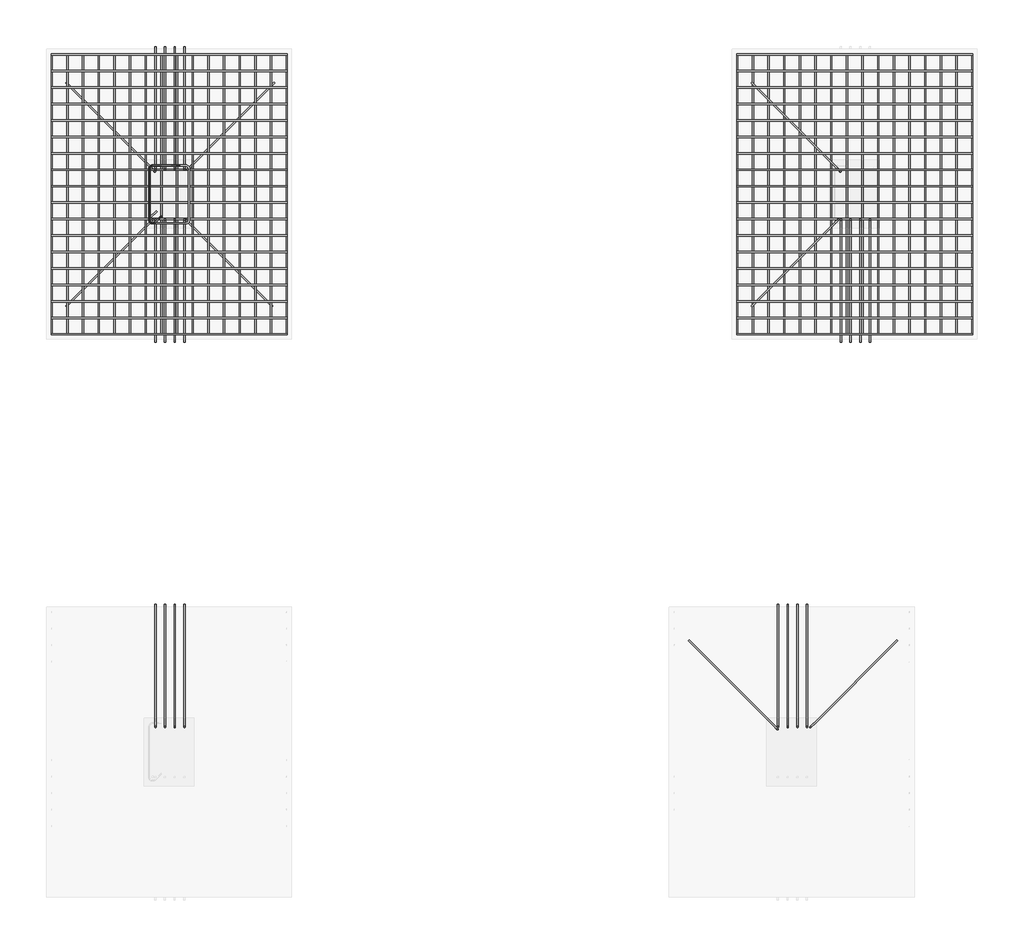
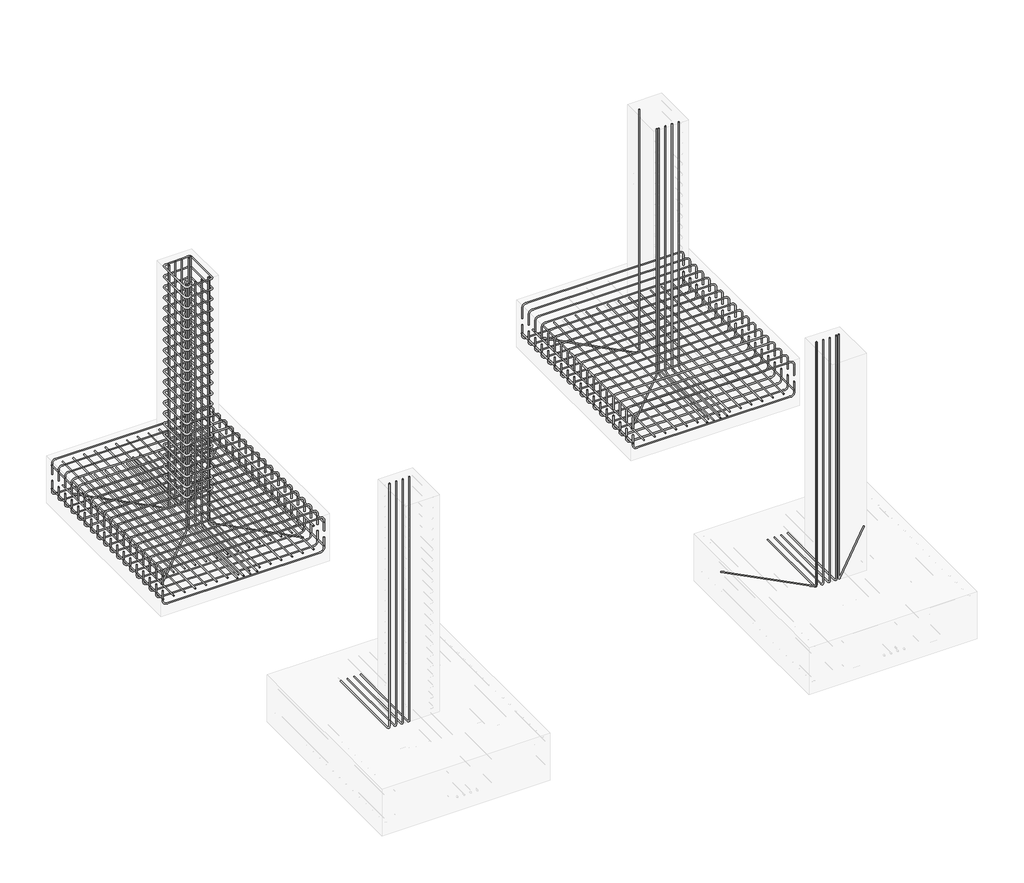
# One storey, part 12 of 33: 21 reinforcing bars.
"""IFC4 building model written with IfcOpenShell, lengths in millimetres."""

from ifc_helpers import new_model, si_unit, point, frame, origin, place, context, project, spatial, polyline, circle_curve, trimmed, segment, composite_curve, source, transform, mapped, element, save
from ifc_brep_helpers import swept_disk

model = new_model("IFC4")

# Units and contexts
model_context = context("Model", 3, world=origin())
ifc_project = project(units=[si_unit("LENGTHUNIT", "METRE", prefix="MILLI")], contexts=[model_context])

# Site, building, storey
site = spatial("IfcSite", under=ifc_project)
building = spatial("IfcBuilding", under=site)
storey = spatial("IfcBuildingStorey", under=building, Elevation=-3000.0)

# Reinforcing bars
placement = place(None, origin())
reinforcing_bar_shape = source(origin(), model_context, "Body", "SolidModel", [
    swept_disk(composite_curve([segment(polyline([(25452.7737106, -2044.0608134, -3240.0), (25452.7737106, -2044.0608134, -3092.7)]), True, "CONTINUOUS"), segment(trimmed(circle_curve(frame((25499.1237106, -2044.0608134, -3092.7), z_axis=(0.0, 1.0, 0.0), x_axis=(-46.35000000000218, 0.0, 0.0)), 46.35), [point((25452.7737106, -2044.0608134, -3092.7))], [point((25499.1237106, -2044.0608134, -3046.35))], True, "CARTESIAN"), True, "CONTINUOUS"), segment(polyline([(25499.1237106, -2044.0608134, -3046.35), (27513.7237106, -2044.0608134, -3046.35)]), True, "CONTINUOUS"), segment(trimmed(circle_curve(frame((27513.7237106, -2044.0608134, -3092.7), z_axis=(0.0, 1.0, 0.0), x_axis=(0.0, 0.0, 46.34999999999991)), 46.35), [point((27513.7237106, -2044.0608134, -3046.35))], [point((27560.0737106, -2044.0608134, -3092.7))], True, "CARTESIAN"), True, "CONTINUOUS"), segment(polyline([(27560.0737106, -2044.0608134, -3092.7), (27560.0737106, -2044.0608134, -3240.0)]), True, "CONTINUOUS")], self_intersect=False), 6.35),
])
element("IfcReinforcingBar", 1, at=placement, inside=storey, context=model_context, shape_type="MappedRepresentation", body=[
    mapped(reinforcing_bar_shape, transform((0.0, 0.0, 0.0), x_axis=(1.0, 0.0, 0.0), y_axis=(0.0, 1.0, 0.0), z_axis=(0.0, 0.0, 1.0))),
    mapped(reinforcing_bar_shape, transform((0.0, -147.4882353, 0.0), x_axis=(1.0, 0.0, 0.0), y_axis=(0.0, 1.0, 0.0), z_axis=(0.0, 0.0, 1.0))),
    mapped(reinforcing_bar_shape, transform((0.0, -294.9764706, 0.0), x_axis=(1.0, 0.0, 0.0), y_axis=(0.0, 1.0, 0.0), z_axis=(0.0, 0.0, 1.0))),
    mapped(reinforcing_bar_shape, transform((0.0, -442.4647059, 0.0), x_axis=(1.0, 0.0, 0.0), y_axis=(0.0, 1.0, 0.0), z_axis=(0.0, 0.0, 1.0))),
    mapped(reinforcing_bar_shape, transform((0.0, -589.9529412, 0.0), x_axis=(1.0, 0.0, 0.0), y_axis=(0.0, 1.0, 0.0), z_axis=(0.0, 0.0, 1.0))),
    mapped(reinforcing_bar_shape, transform((0.0, -737.4411765, 0.0), x_axis=(1.0, 0.0, 0.0), y_axis=(0.0, 1.0, 0.0), z_axis=(0.0, 0.0, 1.0))),
    mapped(reinforcing_bar_shape, transform((0.0, -884.9294118, 0.0), x_axis=(1.0, 0.0, 0.0), y_axis=(0.0, 1.0, 0.0), z_axis=(0.0, 0.0, 1.0))),
    mapped(reinforcing_bar_shape, transform((0.0, -1032.4176471, 0.0), x_axis=(1.0, 0.0, 0.0), y_axis=(0.0, 1.0, 0.0), z_axis=(0.0, 0.0, 1.0))),
    mapped(reinforcing_bar_shape, transform((0.0, -1179.9058824, 0.0), x_axis=(1.0, 0.0, 0.0), y_axis=(0.0, 1.0, 0.0), z_axis=(0.0, 0.0, 1.0))),
    mapped(reinforcing_bar_shape, transform((0.0, -1327.3941176, 0.0), x_axis=(1.0, 0.0, 0.0), y_axis=(0.0, 1.0, 0.0), z_axis=(0.0, 0.0, 1.0))),
    mapped(reinforcing_bar_shape, transform((0.0, -1474.8823529, 0.0), x_axis=(1.0, 0.0, 0.0), y_axis=(0.0, 1.0, 0.0), z_axis=(0.0, 0.0, 1.0))),
    mapped(reinforcing_bar_shape, transform((0.0, -1622.3705882, 0.0), x_axis=(1.0, 0.0, 0.0), y_axis=(0.0, 1.0, 0.0), z_axis=(0.0, 0.0, 1.0))),
    mapped(reinforcing_bar_shape, transform((0.0, -1769.8588235, 0.0), x_axis=(1.0, 0.0, 0.0), y_axis=(0.0, 1.0, 0.0), z_axis=(0.0, 0.0, 1.0))),
    mapped(reinforcing_bar_shape, transform((0.0, -1917.3470588, 0.0), x_axis=(1.0, 0.0, 0.0), y_axis=(0.0, 1.0, 0.0), z_axis=(0.0, 0.0, 1.0))),
    mapped(reinforcing_bar_shape, transform((0.0, -2064.8352941, 0.0), x_axis=(1.0, 0.0, 0.0), y_axis=(0.0, 1.0, 0.0), z_axis=(0.0, 0.0, 1.0))),
    mapped(reinforcing_bar_shape, transform((0.0, -2212.3235294, 0.0), x_axis=(1.0, 0.0, 0.0), y_axis=(0.0, 1.0, 0.0), z_axis=(0.0, 0.0, 1.0))),
    mapped(reinforcing_bar_shape, transform((0.0, -2359.8117647, 0.0), x_axis=(1.0, 0.0, 0.0), y_axis=(0.0, 1.0, 0.0), z_axis=(0.0, 0.0, 1.0))),
    mapped(reinforcing_bar_shape, transform((0.0, -2507.3, 0.0), x_axis=(1.0, 0.0, 0.0), y_axis=(0.0, 1.0, 0.0), z_axis=(0.0, 0.0, 1.0))),
])
reinforcing_bar_2_shape = source(origin(), model_context, "Body", "SolidModel", [
    swept_disk(composite_curve([segment(polyline([(27560.0737106, -2044.0608134, -3330.080452), (27560.0737106, -2044.0608134, -3477.380452)]), True, "CONTINUOUS"), segment(trimmed(circle_curve(frame((27513.7237106, -2044.0608134, -3477.380452), z_axis=(0.0, 1.0, 0.0), x_axis=(46.35000000000218, 0.0, 0.0)), 46.35), [point((27560.0737106, -2044.0608134, -3477.380452))], [point((27513.7237106, -2044.0608134, -3523.730452))], True, "CARTESIAN"), True, "CONTINUOUS"), segment(polyline([(27513.7237106, -2044.0608134, -3523.730452), (25499.1237106, -2044.0608134, -3523.730452)]), True, "CONTINUOUS"), segment(trimmed(circle_curve(frame((25499.1237106, -2044.0608134, -3477.380452), z_axis=(0.0, 1.0, 0.0), x_axis=(0.0, 0.0, -46.34999999999991)), 46.35), [point((25499.1237106, -2044.0608134, -3523.730452))], [point((25452.7737106, -2044.0608134, -3477.380452))], True, "CARTESIAN"), True, "CONTINUOUS"), segment(polyline([(25452.7737106, -2044.0608134, -3477.380452), (25452.7737106, -2044.0608134, -3330.080452)]), True, "CONTINUOUS")], self_intersect=False), 6.35),
])
element("IfcReinforcingBar", 2, at=placement, inside=storey, context=model_context, shape_type="MappedRepresentation", body=[
    mapped(reinforcing_bar_2_shape, transform((0.0, 0.0, 0.0), x_axis=(1.0, 0.0, 0.0), y_axis=(0.0, 1.0, 0.0), z_axis=(0.0, 0.0, 1.0))),
    mapped(reinforcing_bar_2_shape, transform((0.0, -147.4882353, 0.0), x_axis=(1.0, 0.0, 0.0), y_axis=(0.0, 1.0, 0.0), z_axis=(0.0, 0.0, 1.0))),
    mapped(reinforcing_bar_2_shape, transform((0.0, -294.9764706, 0.0), x_axis=(1.0, 0.0, 0.0), y_axis=(0.0, 1.0, 0.0), z_axis=(0.0, 0.0, 1.0))),
    mapped(reinforcing_bar_2_shape, transform((0.0, -442.4647059, 0.0), x_axis=(1.0, 0.0, 0.0), y_axis=(0.0, 1.0, 0.0), z_axis=(0.0, 0.0, 1.0))),
    mapped(reinforcing_bar_2_shape, transform((0.0, -589.9529412, 0.0), x_axis=(1.0, 0.0, 0.0), y_axis=(0.0, 1.0, 0.0), z_axis=(0.0, 0.0, 1.0))),
    mapped(reinforcing_bar_2_shape, transform((0.0, -737.4411765, 0.0), x_axis=(1.0, 0.0, 0.0), y_axis=(0.0, 1.0, 0.0), z_axis=(0.0, 0.0, 1.0))),
    mapped(reinforcing_bar_2_shape, transform((0.0, -884.9294118, 0.0), x_axis=(1.0, 0.0, 0.0), y_axis=(0.0, 1.0, 0.0), z_axis=(0.0, 0.0, 1.0))),
    mapped(reinforcing_bar_2_shape, transform((0.0, -1032.4176471, 0.0), x_axis=(1.0, 0.0, 0.0), y_axis=(0.0, 1.0, 0.0), z_axis=(0.0, 0.0, 1.0))),
    mapped(reinforcing_bar_2_shape, transform((0.0, -1179.9058824, 0.0), x_axis=(1.0, 0.0, 0.0), y_axis=(0.0, 1.0, 0.0), z_axis=(0.0, 0.0, 1.0))),
    mapped(reinforcing_bar_2_shape, transform((0.0, -1327.3941176, 0.0), x_axis=(1.0, 0.0, 0.0), y_axis=(0.0, 1.0, 0.0), z_axis=(0.0, 0.0, 1.0))),
    mapped(reinforcing_bar_2_shape, transform((0.0, -1474.8823529, 0.0), x_axis=(1.0, 0.0, 0.0), y_axis=(0.0, 1.0, 0.0), z_axis=(0.0, 0.0, 1.0))),
    mapped(reinforcing_bar_2_shape, transform((0.0, -1622.3705882, 0.0), x_axis=(1.0, 0.0, 0.0), y_axis=(0.0, 1.0, 0.0), z_axis=(0.0, 0.0, 1.0))),
    mapped(reinforcing_bar_2_shape, transform((0.0, -1769.8588235, 0.0), x_axis=(1.0, 0.0, 0.0), y_axis=(0.0, 1.0, 0.0), z_axis=(0.0, 0.0, 1.0))),
    mapped(reinforcing_bar_2_shape, transform((0.0, -1917.3470588, 0.0), x_axis=(1.0, 0.0, 0.0), y_axis=(0.0, 1.0, 0.0), z_axis=(0.0, 0.0, 1.0))),
    mapped(reinforcing_bar_2_shape, transform((0.0, -2064.8352941, 0.0), x_axis=(1.0, 0.0, 0.0), y_axis=(0.0, 1.0, 0.0), z_axis=(0.0, 0.0, 1.0))),
    mapped(reinforcing_bar_2_shape, transform((0.0, -2212.3235294, 0.0), x_axis=(1.0, 0.0, 0.0), y_axis=(0.0, 1.0, 0.0), z_axis=(0.0, 0.0, 1.0))),
    mapped(reinforcing_bar_2_shape, transform((0.0, -2359.8117647, 0.0), x_axis=(1.0, 0.0, 0.0), y_axis=(0.0, 1.0, 0.0), z_axis=(0.0, 0.0, 1.0))),
    mapped(reinforcing_bar_2_shape, transform((0.0, -2507.3, 0.0), x_axis=(1.0, 0.0, 0.0), y_axis=(0.0, 1.0, 0.0), z_axis=(0.0, 0.0, 1.0))),
])
reinforcing_bar_3_shape = source(origin(), model_context, "Body", "SolidModel", [
    swept_disk(composite_curve([segment(polyline([(27560.0737106, -4557.7108134, -3447.8614173), (27560.0737106, -2037.7108134, -3447.8614173)]), True, "CONTINUOUS")], self_intersect=False), 6.35),
])
element("IfcReinforcingBar", 3, at=placement, inside=storey, context=model_context, shape_type="MappedRepresentation", body=[
    mapped(reinforcing_bar_3_shape, transform((0.0, 0.0, 0.0), x_axis=(1.0, 0.0, 0.0), y_axis=(0.0, 1.0, 0.0), z_axis=(0.0, 0.0, 1.0))),
    mapped(reinforcing_bar_3_shape, transform((-140.4866667, 0.0, 0.0), x_axis=(1.0, 0.0, 0.0), y_axis=(0.0, 1.0, 0.0), z_axis=(0.0, 0.0, 1.0))),
    mapped(reinforcing_bar_3_shape, transform((-280.9733333, 0.0, 0.0), x_axis=(1.0, 0.0, 0.0), y_axis=(0.0, 1.0, 0.0), z_axis=(0.0, 0.0, 1.0))),
    mapped(reinforcing_bar_3_shape, transform((-421.46, 0.0, 0.0), x_axis=(1.0, 0.0, 0.0), y_axis=(0.0, 1.0, 0.0), z_axis=(0.0, 0.0, 1.0))),
    mapped(reinforcing_bar_3_shape, transform((-561.9466667, 0.0, 0.0), x_axis=(1.0, 0.0, 0.0), y_axis=(0.0, 1.0, 0.0), z_axis=(0.0, 0.0, 1.0))),
    mapped(reinforcing_bar_3_shape, transform((-702.4333333, 0.0, 0.0), x_axis=(1.0, 0.0, 0.0), y_axis=(0.0, 1.0, 0.0), z_axis=(0.0, 0.0, 1.0))),
    mapped(reinforcing_bar_3_shape, transform((-842.92, 0.0, 0.0), x_axis=(1.0, 0.0, 0.0), y_axis=(0.0, 1.0, 0.0), z_axis=(0.0, 0.0, 1.0))),
    mapped(reinforcing_bar_3_shape, transform((-983.4066667, 0.0, 0.0), x_axis=(1.0, 0.0, 0.0), y_axis=(0.0, 1.0, 0.0), z_axis=(0.0, 0.0, 1.0))),
    mapped(reinforcing_bar_3_shape, transform((-1123.8933333, 0.0, 0.0), x_axis=(1.0, 0.0, 0.0), y_axis=(0.0, 1.0, 0.0), z_axis=(0.0, 0.0, 1.0))),
    mapped(reinforcing_bar_3_shape, transform((-1264.38, 0.0, 0.0), x_axis=(1.0, 0.0, 0.0), y_axis=(0.0, 1.0, 0.0), z_axis=(0.0, 0.0, 1.0))),
    mapped(reinforcing_bar_3_shape, transform((-1404.8666667, 0.0, 0.0), x_axis=(1.0, 0.0, 0.0), y_axis=(0.0, 1.0, 0.0), z_axis=(0.0, 0.0, 1.0))),
    mapped(reinforcing_bar_3_shape, transform((-1545.3533333, 0.0, 0.0), x_axis=(1.0, 0.0, 0.0), y_axis=(0.0, 1.0, 0.0), z_axis=(0.0, 0.0, 1.0))),
    mapped(reinforcing_bar_3_shape, transform((-1685.84, 0.0, 0.0), x_axis=(1.0, 0.0, 0.0), y_axis=(0.0, 1.0, 0.0), z_axis=(0.0, 0.0, 1.0))),
    mapped(reinforcing_bar_3_shape, transform((-1826.3266667, 0.0, 0.0), x_axis=(1.0, 0.0, 0.0), y_axis=(0.0, 1.0, 0.0), z_axis=(0.0, 0.0, 1.0))),
    mapped(reinforcing_bar_3_shape, transform((-1966.8133333, 0.0, 0.0), x_axis=(1.0, 0.0, 0.0), y_axis=(0.0, 1.0, 0.0), z_axis=(0.0, 0.0, 1.0))),
    mapped(reinforcing_bar_3_shape, transform((-2107.3, 0.0, 0.0), x_axis=(1.0, 0.0, 0.0), y_axis=(0.0, 1.0, 0.0), z_axis=(0.0, 0.0, 1.0))),
])
reinforcing_bar_4_shape = source(origin(), model_context, "Body", "SolidModel", [
    swept_disk(composite_curve([segment(polyline([(19306.5357258, -2044.0608134, -3240.0), (19306.5357258, -2044.0608134, -3092.7)]), True, "CONTINUOUS"), segment(trimmed(circle_curve(frame((19352.8857258, -2044.0608134, -3092.7), z_axis=(0.0, 1.0, 0.0), x_axis=(-46.349999999998545, 0.0, 0.0)), 46.35), [point((19306.5357258, -2044.0608134, -3092.7))], [point((19352.8857258, -2044.0608134, -3046.35))], True, "CARTESIAN"), True, "CONTINUOUS"), segment(polyline([(19352.8857258, -2044.0608134, -3046.35), (21367.4857258, -2044.0608134, -3046.35)]), True, "CONTINUOUS"), segment(trimmed(circle_curve(frame((21367.4857258, -2044.0608134, -3092.7), z_axis=(0.0, 1.0, 0.0), x_axis=(0.0, 0.0, 46.34999999999991)), 46.35), [point((21367.4857258, -2044.0608134, -3046.35))], [point((21413.8357258, -2044.0608134, -3092.7))], True, "CARTESIAN"), True, "CONTINUOUS"), segment(polyline([(21413.8357258, -2044.0608134, -3092.7), (21413.8357258, -2044.0608134, -3240.0)]), True, "CONTINUOUS")], self_intersect=False), 6.35),
])
element("IfcReinforcingBar", 4, at=placement, inside=storey, context=model_context, shape_type="MappedRepresentation", body=[
    mapped(reinforcing_bar_4_shape, transform((0.0, 0.0, 0.0), x_axis=(1.0, 0.0, 0.0), y_axis=(0.0, 1.0, 0.0), z_axis=(0.0, 0.0, 1.0))),
    mapped(reinforcing_bar_4_shape, transform((0.0, -147.4882353, 0.0), x_axis=(1.0, 0.0, 0.0), y_axis=(0.0, 1.0, 0.0), z_axis=(0.0, 0.0, 1.0))),
    mapped(reinforcing_bar_4_shape, transform((0.0, -294.9764706, 0.0), x_axis=(1.0, 0.0, 0.0), y_axis=(0.0, 1.0, 0.0), z_axis=(0.0, 0.0, 1.0))),
    mapped(reinforcing_bar_4_shape, transform((0.0, -442.4647059, 0.0), x_axis=(1.0, 0.0, 0.0), y_axis=(0.0, 1.0, 0.0), z_axis=(0.0, 0.0, 1.0))),
    mapped(reinforcing_bar_4_shape, transform((0.0, -589.9529412, 0.0), x_axis=(1.0, 0.0, 0.0), y_axis=(0.0, 1.0, 0.0), z_axis=(0.0, 0.0, 1.0))),
    mapped(reinforcing_bar_4_shape, transform((0.0, -737.4411765, 0.0), x_axis=(1.0, 0.0, 0.0), y_axis=(0.0, 1.0, 0.0), z_axis=(0.0, 0.0, 1.0))),
    mapped(reinforcing_bar_4_shape, transform((0.0, -884.9294118, 0.0), x_axis=(1.0, 0.0, 0.0), y_axis=(0.0, 1.0, 0.0), z_axis=(0.0, 0.0, 1.0))),
    mapped(reinforcing_bar_4_shape, transform((0.0, -1032.4176471, 0.0), x_axis=(1.0, 0.0, 0.0), y_axis=(0.0, 1.0, 0.0), z_axis=(0.0, 0.0, 1.0))),
    mapped(reinforcing_bar_4_shape, transform((0.0, -1179.9058824, 0.0), x_axis=(1.0, 0.0, 0.0), y_axis=(0.0, 1.0, 0.0), z_axis=(0.0, 0.0, 1.0))),
    mapped(reinforcing_bar_4_shape, transform((0.0, -1327.3941176, 0.0), x_axis=(1.0, 0.0, 0.0), y_axis=(0.0, 1.0, 0.0), z_axis=(0.0, 0.0, 1.0))),
    mapped(reinforcing_bar_4_shape, transform((0.0, -1474.8823529, 0.0), x_axis=(1.0, 0.0, 0.0), y_axis=(0.0, 1.0, 0.0), z_axis=(0.0, 0.0, 1.0))),
    mapped(reinforcing_bar_4_shape, transform((0.0, -1622.3705882, 0.0), x_axis=(1.0, 0.0, 0.0), y_axis=(0.0, 1.0, 0.0), z_axis=(0.0, 0.0, 1.0))),
    mapped(reinforcing_bar_4_shape, transform((0.0, -1769.8588235, 0.0), x_axis=(1.0, 0.0, 0.0), y_axis=(0.0, 1.0, 0.0), z_axis=(0.0, 0.0, 1.0))),
    mapped(reinforcing_bar_4_shape, transform((0.0, -1917.3470588, 0.0), x_axis=(1.0, 0.0, 0.0), y_axis=(0.0, 1.0, 0.0), z_axis=(0.0, 0.0, 1.0))),
    mapped(reinforcing_bar_4_shape, transform((0.0, -2064.8352941, 0.0), x_axis=(1.0, 0.0, 0.0), y_axis=(0.0, 1.0, 0.0), z_axis=(0.0, 0.0, 1.0))),
    mapped(reinforcing_bar_4_shape, transform((0.0, -2212.3235294, 0.0), x_axis=(1.0, 0.0, 0.0), y_axis=(0.0, 1.0, 0.0), z_axis=(0.0, 0.0, 1.0))),
    mapped(reinforcing_bar_4_shape, transform((0.0, -2359.8117647, 0.0), x_axis=(1.0, 0.0, 0.0), y_axis=(0.0, 1.0, 0.0), z_axis=(0.0, 0.0, 1.0))),
    mapped(reinforcing_bar_4_shape, transform((0.0, -2507.3, 0.0), x_axis=(1.0, 0.0, 0.0), y_axis=(0.0, 1.0, 0.0), z_axis=(0.0, 0.0, 1.0))),
])
reinforcing_bar_5_shape = source(origin(), model_context, "Body", "SolidModel", [
    swept_disk(composite_curve([segment(polyline([(21413.8357258, -2044.0608134, -3330.080452), (21413.8357258, -2044.0608134, -3477.380452)]), True, "CONTINUOUS"), segment(trimmed(circle_curve(frame((21367.4857258, -2044.0608134, -3477.380452), z_axis=(0.0, 1.0, 0.0), x_axis=(46.349999999998545, 0.0, 0.0)), 46.35), [point((21413.8357258, -2044.0608134, -3477.380452))], [point((21367.4857258, -2044.0608134, -3523.730452))], True, "CARTESIAN"), True, "CONTINUOUS"), segment(polyline([(21367.4857258, -2044.0608134, -3523.730452), (19352.8857258, -2044.0608134, -3523.730452)]), True, "CONTINUOUS"), segment(trimmed(circle_curve(frame((19352.8857258, -2044.0608134, -3477.380452), z_axis=(0.0, 1.0, 0.0), x_axis=(0.0, 0.0, -46.34999999999991)), 46.35), [point((19352.8857258, -2044.0608134, -3523.730452))], [point((19306.5357258, -2044.0608134, -3477.380452))], True, "CARTESIAN"), True, "CONTINUOUS"), segment(polyline([(19306.5357258, -2044.0608134, -3477.380452), (19306.5357258, -2044.0608134, -3330.080452)]), True, "CONTINUOUS")], self_intersect=False), 6.35),
])
element("IfcReinforcingBar", 5, at=placement, inside=storey, context=model_context, shape_type="MappedRepresentation", body=[
    mapped(reinforcing_bar_5_shape, transform((0.0, 0.0, 0.0), x_axis=(1.0, 0.0, 0.0), y_axis=(0.0, 1.0, 0.0), z_axis=(0.0, 0.0, 1.0))),
    mapped(reinforcing_bar_5_shape, transform((0.0, -147.4882353, 0.0), x_axis=(1.0, 0.0, 0.0), y_axis=(0.0, 1.0, 0.0), z_axis=(0.0, 0.0, 1.0))),
    mapped(reinforcing_bar_5_shape, transform((0.0, -294.9764706, 0.0), x_axis=(1.0, 0.0, 0.0), y_axis=(0.0, 1.0, 0.0), z_axis=(0.0, 0.0, 1.0))),
    mapped(reinforcing_bar_5_shape, transform((0.0, -442.4647059, 0.0), x_axis=(1.0, 0.0, 0.0), y_axis=(0.0, 1.0, 0.0), z_axis=(0.0, 0.0, 1.0))),
    mapped(reinforcing_bar_5_shape, transform((0.0, -589.9529412, 0.0), x_axis=(1.0, 0.0, 0.0), y_axis=(0.0, 1.0, 0.0), z_axis=(0.0, 0.0, 1.0))),
    mapped(reinforcing_bar_5_shape, transform((0.0, -737.4411765, 0.0), x_axis=(1.0, 0.0, 0.0), y_axis=(0.0, 1.0, 0.0), z_axis=(0.0, 0.0, 1.0))),
    mapped(reinforcing_bar_5_shape, transform((0.0, -884.9294118, 0.0), x_axis=(1.0, 0.0, 0.0), y_axis=(0.0, 1.0, 0.0), z_axis=(0.0, 0.0, 1.0))),
    mapped(reinforcing_bar_5_shape, transform((0.0, -1032.4176471, 0.0), x_axis=(1.0, 0.0, 0.0), y_axis=(0.0, 1.0, 0.0), z_axis=(0.0, 0.0, 1.0))),
    mapped(reinforcing_bar_5_shape, transform((0.0, -1179.9058824, 0.0), x_axis=(1.0, 0.0, 0.0), y_axis=(0.0, 1.0, 0.0), z_axis=(0.0, 0.0, 1.0))),
    mapped(reinforcing_bar_5_shape, transform((0.0, -1327.3941176, 0.0), x_axis=(1.0, 0.0, 0.0), y_axis=(0.0, 1.0, 0.0), z_axis=(0.0, 0.0, 1.0))),
    mapped(reinforcing_bar_5_shape, transform((0.0, -1474.8823529, 0.0), x_axis=(1.0, 0.0, 0.0), y_axis=(0.0, 1.0, 0.0), z_axis=(0.0, 0.0, 1.0))),
    mapped(reinforcing_bar_5_shape, transform((0.0, -1622.3705882, 0.0), x_axis=(1.0, 0.0, 0.0), y_axis=(0.0, 1.0, 0.0), z_axis=(0.0, 0.0, 1.0))),
    mapped(reinforcing_bar_5_shape, transform((0.0, -1769.8588235, 0.0), x_axis=(1.0, 0.0, 0.0), y_axis=(0.0, 1.0, 0.0), z_axis=(0.0, 0.0, 1.0))),
    mapped(reinforcing_bar_5_shape, transform((0.0, -1917.3470588, 0.0), x_axis=(1.0, 0.0, 0.0), y_axis=(0.0, 1.0, 0.0), z_axis=(0.0, 0.0, 1.0))),
    mapped(reinforcing_bar_5_shape, transform((0.0, -2064.8352941, 0.0), x_axis=(1.0, 0.0, 0.0), y_axis=(0.0, 1.0, 0.0), z_axis=(0.0, 0.0, 1.0))),
    mapped(reinforcing_bar_5_shape, transform((0.0, -2212.3235294, 0.0), x_axis=(1.0, 0.0, 0.0), y_axis=(0.0, 1.0, 0.0), z_axis=(0.0, 0.0, 1.0))),
    mapped(reinforcing_bar_5_shape, transform((0.0, -2359.8117647, 0.0), x_axis=(1.0, 0.0, 0.0), y_axis=(0.0, 1.0, 0.0), z_axis=(0.0, 0.0, 1.0))),
    mapped(reinforcing_bar_5_shape, transform((0.0, -2507.3, 0.0), x_axis=(1.0, 0.0, 0.0), y_axis=(0.0, 1.0, 0.0), z_axis=(0.0, 0.0, 1.0))),
])
reinforcing_bar_6_shape = source(origin(), model_context, "Body", "SolidModel", [
    swept_disk(composite_curve([segment(polyline([(21413.8357258, -4557.7108134, -3447.8614173), (21413.8357258, -2037.7108134, -3447.8614173)]), True, "CONTINUOUS")], self_intersect=False), 6.35),
])
element("IfcReinforcingBar", 6, at=placement, inside=storey, context=model_context, shape_type="MappedRepresentation", body=[
    mapped(reinforcing_bar_6_shape, transform((0.0, 0.0, 0.0), x_axis=(1.0, 0.0, 0.0), y_axis=(0.0, 1.0, 0.0), z_axis=(0.0, 0.0, 1.0))),
    mapped(reinforcing_bar_6_shape, transform((-140.4866667, 0.0, 0.0), x_axis=(1.0, 0.0, 0.0), y_axis=(0.0, 1.0, 0.0), z_axis=(0.0, 0.0, 1.0))),
    mapped(reinforcing_bar_6_shape, transform((-280.9733333, 0.0, 0.0), x_axis=(1.0, 0.0, 0.0), y_axis=(0.0, 1.0, 0.0), z_axis=(0.0, 0.0, 1.0))),
    mapped(reinforcing_bar_6_shape, transform((-421.46, 0.0, 0.0), x_axis=(1.0, 0.0, 0.0), y_axis=(0.0, 1.0, 0.0), z_axis=(0.0, 0.0, 1.0))),
    mapped(reinforcing_bar_6_shape, transform((-561.9466667, 0.0, 0.0), x_axis=(1.0, 0.0, 0.0), y_axis=(0.0, 1.0, 0.0), z_axis=(0.0, 0.0, 1.0))),
    mapped(reinforcing_bar_6_shape, transform((-702.4333333, 0.0, 0.0), x_axis=(1.0, 0.0, 0.0), y_axis=(0.0, 1.0, 0.0), z_axis=(0.0, 0.0, 1.0))),
    mapped(reinforcing_bar_6_shape, transform((-842.92, 0.0, 0.0), x_axis=(1.0, 0.0, 0.0), y_axis=(0.0, 1.0, 0.0), z_axis=(0.0, 0.0, 1.0))),
    mapped(reinforcing_bar_6_shape, transform((-983.4066667, 0.0, 0.0), x_axis=(1.0, 0.0, 0.0), y_axis=(0.0, 1.0, 0.0), z_axis=(0.0, 0.0, 1.0))),
    mapped(reinforcing_bar_6_shape, transform((-1123.8933333, 0.0, 0.0), x_axis=(1.0, 0.0, 0.0), y_axis=(0.0, 1.0, 0.0), z_axis=(0.0, 0.0, 1.0))),
    mapped(reinforcing_bar_6_shape, transform((-1264.38, 0.0, 0.0), x_axis=(1.0, 0.0, 0.0), y_axis=(0.0, 1.0, 0.0), z_axis=(0.0, 0.0, 1.0))),
    mapped(reinforcing_bar_6_shape, transform((-1404.8666667, 0.0, 0.0), x_axis=(1.0, 0.0, 0.0), y_axis=(0.0, 1.0, 0.0), z_axis=(0.0, 0.0, 1.0))),
    mapped(reinforcing_bar_6_shape, transform((-1545.3533333, 0.0, 0.0), x_axis=(1.0, 0.0, 0.0), y_axis=(0.0, 1.0, 0.0), z_axis=(0.0, 0.0, 1.0))),
    mapped(reinforcing_bar_6_shape, transform((-1685.84, 0.0, 0.0), x_axis=(1.0, 0.0, 0.0), y_axis=(0.0, 1.0, 0.0), z_axis=(0.0, 0.0, 1.0))),
    mapped(reinforcing_bar_6_shape, transform((-1826.3266667, 0.0, 0.0), x_axis=(1.0, 0.0, 0.0), y_axis=(0.0, 1.0, 0.0), z_axis=(0.0, 0.0, 1.0))),
    mapped(reinforcing_bar_6_shape, transform((-1966.8133333, 0.0, 0.0), x_axis=(1.0, 0.0, 0.0), y_axis=(0.0, 1.0, 0.0), z_axis=(0.0, 0.0, 1.0))),
    mapped(reinforcing_bar_6_shape, transform((-2107.3, 0.0, 0.0), x_axis=(1.0, 0.0, 0.0), y_axis=(0.0, 1.0, 0.0), z_axis=(0.0, 0.0, 1.0))),
])
reinforcing_bar_7_shape = source(origin(), model_context, "Body", "SolidModel", [
    swept_disk(composite_curve([segment(polyline([(19306.5357258, -4557.7108134, -3122.7084113), (19306.5357258, -2037.7108134, -3122.7084113)]), True, "CONTINUOUS")], self_intersect=False), 6.35),
])
element("IfcReinforcingBar", 7, at=placement, inside=storey, context=model_context, shape_type="MappedRepresentation", body=[
    mapped(reinforcing_bar_7_shape, transform((0.0, 0.0, 0.0), x_axis=(1.0, 0.0, 0.0), y_axis=(0.0, 1.0, 0.0), z_axis=(0.0, 0.0, 1.0))),
    mapped(reinforcing_bar_7_shape, transform((140.4866667, 0.0, 0.0), x_axis=(1.0, 0.0, 0.0), y_axis=(0.0, 1.0, 0.0), z_axis=(0.0, 0.0, 1.0))),
    mapped(reinforcing_bar_7_shape, transform((280.9733333, 0.0, 0.0), x_axis=(1.0, 0.0, 0.0), y_axis=(0.0, 1.0, 0.0), z_axis=(0.0, 0.0, 1.0))),
    mapped(reinforcing_bar_7_shape, transform((421.46, 0.0, 0.0), x_axis=(1.0, 0.0, 0.0), y_axis=(0.0, 1.0, 0.0), z_axis=(0.0, 0.0, 1.0))),
    mapped(reinforcing_bar_7_shape, transform((561.9466667, 0.0, 0.0), x_axis=(1.0, 0.0, 0.0), y_axis=(0.0, 1.0, 0.0), z_axis=(0.0, 0.0, 1.0))),
    mapped(reinforcing_bar_7_shape, transform((702.4333333, 0.0, 0.0), x_axis=(1.0, 0.0, 0.0), y_axis=(0.0, 1.0, 0.0), z_axis=(0.0, 0.0, 1.0))),
    mapped(reinforcing_bar_7_shape, transform((842.92, 0.0, 0.0), x_axis=(1.0, 0.0, 0.0), y_axis=(0.0, 1.0, 0.0), z_axis=(0.0, 0.0, 1.0))),
    mapped(reinforcing_bar_7_shape, transform((983.4066667, 0.0, 0.0), x_axis=(1.0, 0.0, 0.0), y_axis=(0.0, 1.0, 0.0), z_axis=(0.0, 0.0, 1.0))),
    mapped(reinforcing_bar_7_shape, transform((1123.8933333, 0.0, 0.0), x_axis=(1.0, 0.0, 0.0), y_axis=(0.0, 1.0, 0.0), z_axis=(0.0, 0.0, 1.0))),
    mapped(reinforcing_bar_7_shape, transform((1264.38, 0.0, 0.0), x_axis=(1.0, 0.0, 0.0), y_axis=(0.0, 1.0, 0.0), z_axis=(0.0, 0.0, 1.0))),
    mapped(reinforcing_bar_7_shape, transform((1404.8666667, 0.0, 0.0), x_axis=(1.0, 0.0, 0.0), y_axis=(0.0, 1.0, 0.0), z_axis=(0.0, 0.0, 1.0))),
    mapped(reinforcing_bar_7_shape, transform((1545.3533333, 0.0, 0.0), x_axis=(1.0, 0.0, 0.0), y_axis=(0.0, 1.0, 0.0), z_axis=(0.0, 0.0, 1.0))),
    mapped(reinforcing_bar_7_shape, transform((1685.84, 0.0, 0.0), x_axis=(1.0, 0.0, 0.0), y_axis=(0.0, 1.0, 0.0), z_axis=(0.0, 0.0, 1.0))),
    mapped(reinforcing_bar_7_shape, transform((1826.3266667, 0.0, 0.0), x_axis=(1.0, 0.0, 0.0), y_axis=(0.0, 1.0, 0.0), z_axis=(0.0, 0.0, 1.0))),
    mapped(reinforcing_bar_7_shape, transform((1966.8133333, 0.0, 0.0), x_axis=(1.0, 0.0, 0.0), y_axis=(0.0, 1.0, 0.0), z_axis=(0.0, 0.0, 1.0))),
    mapped(reinforcing_bar_7_shape, transform((2107.3, 0.0, 0.0), x_axis=(1.0, 0.0, 0.0), y_axis=(0.0, 1.0, 0.0), z_axis=(0.0, 0.0, 1.0))),
])
reinforcing_bar_8_shape = source(origin(), model_context, "Body", "SolidModel", [
    swept_disk(composite_curve([segment(polyline([(20246.4614911, -3446.8994528, -2953.65), (20190.7179282, -3502.6430158, -2953.65)]), True, "CONTINUOUS"), segment(trimmed(circle_curve(frame((20212.8857258, -3524.8108134, -2953.65), z_axis=(0.0, 0.0, 1.0), x_axis=(-22.167797599999176, 22.167797600000085, 0.0)), 31.35), [point((20190.7179282, -3502.6430158, -2953.65))], [point((20212.8857258, -3556.1608134, -2953.65))], True, "CARTESIAN"), True, "CONTINUOUS"), segment(polyline([(20212.8857258, -3556.1608134, -2953.65), (20507.4857258, -3556.1608134, -2953.65)]), True, "CONTINUOUS"), segment(trimmed(circle_curve(frame((20507.4857258, -3524.8108134, -2953.65), z_axis=(0.0, 0.0, 1.0), x_axis=(0.0, -31.34999999999991, 0.0)), 31.35), [point((20507.4857258, -3556.1608134, -2953.65))], [point((20538.8357258, -3524.8108134, -2953.65))], True, "CARTESIAN"), True, "CONTINUOUS"), segment(polyline([(20538.8357258, -3524.8108134, -2953.65), (20538.8357258, -3070.6108134, -2953.65)]), True, "CONTINUOUS"), segment(trimmed(circle_curve(frame((20507.5055109, -3070.6108134, -2954.7636125), z_axis=(-0.0355219283344822, 0.0, 0.9993688971583016), x_axis=(31.33021490000101, 0.0, 1.1136124999998174)), 31.35), [point((20538.8357258, -3070.6108134, -2953.65))], [point((20507.5055109, -3039.2608134, -2954.7636125))], True, "CARTESIAN"), True, "CONTINUOUS"), segment(polyline([(20507.5055109, -3039.2608134, -2954.7636125), (20212.8659407, -3039.2608134, -2965.2363875)]), True, "CONTINUOUS"), segment(trimmed(circle_curve(frame((20212.8659407, -3070.6108134, -2965.2363875), z_axis=(-0.0355219283344822, 0.0, 0.9993688971583016), x_axis=(0.0, 31.34999999999991, 0.0)), 31.35), [point((20212.8659407, -3039.2608134, -2965.2363875))], [point((20181.5357258, -3070.6108134, -2966.35))], True, "CARTESIAN"), True, "CONTINUOUS"), segment(polyline([(20181.5357258, -3070.6108134, -2966.35), (20181.5357258, -3524.8108134, -2966.35)]), True, "CONTINUOUS"), segment(trimmed(circle_curve(frame((20212.8857258, -3524.8108134, -2966.35), z_axis=(0.0, 0.0, 1.0), x_axis=(-31.349999999998545, 0.0, 0.0)), 31.35), [point((20181.5357258, -3524.8108134, -2966.35))], [point((20235.0535234, -3546.978611, -2966.35))], True, "CARTESIAN"), True, "CONTINUOUS"), segment(polyline([(20235.0535234, -3546.978611, -2966.35), (20290.7970863, -3491.235048, -2966.35)]), True, "CONTINUOUS")], self_intersect=False), 6.35),
])
element("IfcReinforcingBar", 8, at=placement, inside=storey, context=model_context, shape_type="MappedRepresentation", body=[
    mapped(reinforcing_bar_8_shape, transform((0.0, 0.0, 0.0), x_axis=(1.0, 0.0, 0.0), y_axis=(0.0, 1.0, 0.0), z_axis=(0.0, 0.0, 1.0))),
    mapped(reinforcing_bar_8_shape, transform((0.0, 0.0, 145.365), x_axis=(1.0, 0.0, 0.0), y_axis=(0.0, 1.0, 0.0), z_axis=(0.0, 0.0, 1.0))),
    mapped(reinforcing_bar_8_shape, transform((0.0, 0.0, 290.73), x_axis=(1.0, 0.0, 0.0), y_axis=(0.0, 1.0, 0.0), z_axis=(0.0, 0.0, 1.0))),
    mapped(reinforcing_bar_8_shape, transform((0.0, 0.0, 436.095), x_axis=(1.0, 0.0, 0.0), y_axis=(0.0, 1.0, 0.0), z_axis=(0.0, 0.0, 1.0))),
    mapped(reinforcing_bar_8_shape, transform((0.0, 0.0, 581.46), x_axis=(1.0, 0.0, 0.0), y_axis=(0.0, 1.0, 0.0), z_axis=(0.0, 0.0, 1.0))),
    mapped(reinforcing_bar_8_shape, transform((0.0, 0.0, 726.825), x_axis=(1.0, 0.0, 0.0), y_axis=(0.0, 1.0, 0.0), z_axis=(0.0, 0.0, 1.0))),
    mapped(reinforcing_bar_8_shape, transform((0.0, 0.0, 872.19), x_axis=(1.0, 0.0, 0.0), y_axis=(0.0, 1.0, 0.0), z_axis=(0.0, 0.0, 1.0))),
    mapped(reinforcing_bar_8_shape, transform((0.0, 0.0, 1017.555), x_axis=(1.0, 0.0, 0.0), y_axis=(0.0, 1.0, 0.0), z_axis=(0.0, 0.0, 1.0))),
    mapped(reinforcing_bar_8_shape, transform((0.0, 0.0, 1162.92), x_axis=(1.0, 0.0, 0.0), y_axis=(0.0, 1.0, 0.0), z_axis=(0.0, 0.0, 1.0))),
    mapped(reinforcing_bar_8_shape, transform((0.0, 0.0, 1308.285), x_axis=(1.0, 0.0, 0.0), y_axis=(0.0, 1.0, 0.0), z_axis=(0.0, 0.0, 1.0))),
    mapped(reinforcing_bar_8_shape, transform((0.0, 0.0, 1453.65), x_axis=(1.0, 0.0, 0.0), y_axis=(0.0, 1.0, 0.0), z_axis=(0.0, 0.0, 1.0))),
    mapped(reinforcing_bar_8_shape, transform((0.0, 0.0, 1599.015), x_axis=(1.0, 0.0, 0.0), y_axis=(0.0, 1.0, 0.0), z_axis=(0.0, 0.0, 1.0))),
    mapped(reinforcing_bar_8_shape, transform((0.0, 0.0, 1744.38), x_axis=(1.0, 0.0, 0.0), y_axis=(0.0, 1.0, 0.0), z_axis=(0.0, 0.0, 1.0))),
    mapped(reinforcing_bar_8_shape, transform((0.0, 0.0, 1889.745), x_axis=(1.0, 0.0, 0.0), y_axis=(0.0, 1.0, 0.0), z_axis=(0.0, 0.0, 1.0))),
    mapped(reinforcing_bar_8_shape, transform((0.0, 0.0, 2035.11), x_axis=(1.0, 0.0, 0.0), y_axis=(0.0, 1.0, 0.0), z_axis=(0.0, 0.0, 1.0))),
    mapped(reinforcing_bar_8_shape, transform((0.0, 0.0, 2180.475), x_axis=(1.0, 0.0, 0.0), y_axis=(0.0, 1.0, 0.0), z_axis=(0.0, 0.0, 1.0))),
    mapped(reinforcing_bar_8_shape, transform((0.0, 0.0, 2325.84), x_axis=(1.0, 0.0, 0.0), y_axis=(0.0, 1.0, 0.0), z_axis=(0.0, 0.0, 1.0))),
    mapped(reinforcing_bar_8_shape, transform((0.0, 0.0, 2471.205), x_axis=(1.0, 0.0, 0.0), y_axis=(0.0, 1.0, 0.0), z_axis=(0.0, 0.0, 1.0))),
    mapped(reinforcing_bar_8_shape, transform((0.0, 0.0, 2616.57), x_axis=(1.0, 0.0, 0.0), y_axis=(0.0, 1.0, 0.0), z_axis=(0.0, 0.0, 1.0))),
    mapped(reinforcing_bar_8_shape, transform((0.0, 0.0, 2761.935), x_axis=(1.0, 0.0, 0.0), y_axis=(0.0, 1.0, 0.0), z_axis=(0.0, 0.0, 1.0))),
    mapped(reinforcing_bar_8_shape, transform((0.0, 0.0, 2907.3), x_axis=(1.0, 0.0, 0.0), y_axis=(0.0, 1.0, 0.0), z_axis=(0.0, 0.0, 1.0))),
])
element("IfcReinforcingBar", 9, at=placement, inside=storey, context=model_context, shape_type="SolidModel", body=[
    swept_disk(composite_curve([segment(polyline([(20213.2043214, -3521.6339414, -40.0), (20213.2043214, -3521.6339414, -3393.65)]), True, "CONTINUOUS"), segment(trimmed(circle_curve(frame((20180.4299221, -3554.4083407, -3393.65), z_axis=(-0.7071067811865446, 0.7071067811865505, 0.0), x_axis=(32.77439930000037, 32.774399299999914, 0.0)), 46.35), [point((20213.2043214, -3521.6339414, -3393.65))], [point((20180.4299221, -3554.4083407, -3440.0))], True, "CARTESIAN"), True, "CONTINUOUS"), segment(polyline([(20180.4299221, -3554.4083407, -3440.0), (19435.3868621, -4299.4514007, -3440.0)]), True, "CONTINUOUS")], self_intersect=False), 6.35),
])
element("IfcReinforcingBar", 10, at=placement, inside=storey, context=model_context, shape_type="SolidModel", body=[
    swept_disk(composite_curve([segment(polyline([(20231.1024274, -3091.6857913, -40.0), (20231.1024274, -3091.6857913, -3361.434517)]), True, "CONTINUOUS"), segment(trimmed(circle_curve(frame((20198.3280281, -3058.911392, -3361.434517), z_axis=(0.7071067811865539, 0.7071067811865411, 0.0), x_axis=(32.77439930000037, -32.774399299999914, 0.0)), 46.35), [point((20231.1024274, -3091.6857913, -3361.434517))], [point((20198.3280281, -3058.911392, -3407.784517))], True, "CARTESIAN"), True, "CONTINUOUS"), segment(polyline([(20198.3280281, -3058.911392, -3407.784517), (19435.3868621, -2295.970226, -3407.784517)]), True, "CONTINUOUS")], self_intersect=False), 6.35),
])
element("IfcReinforcingBar", 11, at=placement, inside=storey, context=model_context, shape_type="SolidModel", body=[
    swept_disk(composite_curve([segment(polyline([(20507.1671301, -3521.6339414, -40.0), (20507.1671301, -3521.6339414, -3393.65)]), True, "CONTINUOUS"), segment(trimmed(circle_curve(frame((20539.9415294, -3554.4083407, -3393.65), z_axis=(-0.7071067811865493, -0.7071067811865459, 0.0), x_axis=(-32.77439930000037, 32.774399299999914, 0.0)), 46.35), [point((20507.1671301, -3521.6339414, -3393.65))], [point((20539.9415294, -3554.4083407, -3440.0))], True, "CARTESIAN"), True, "CONTINUOUS"), segment(polyline([(20539.9415294, -3554.4083407, -3440.0), (21284.9845894, -4299.4514007, -3440.0)]), True, "CONTINUOUS")], self_intersect=False), 6.35),
])
element("IfcReinforcingBar", 12, at=placement, inside=storey, context=model_context, shape_type="SolidModel", body=[
    swept_disk(composite_curve([segment(polyline([(20525.7684217, -3073.7876853, -30.2564663), (20525.7684217, -3073.7876853, -3383.9064663)]), True, "CONTINUOUS"), segment(trimmed(circle_curve(frame((20558.542821, -3041.013286, -3383.9064663), z_axis=(0.7071067811865493, -0.7071067811865459, 0.0), x_axis=(-32.77439930000037, -32.774399299999914, 0.0)), 46.35), [point((20525.7684217, -3073.7876853, -3383.9064663))], [point((20558.542821, -3041.013286, -3430.2564663))], True, "CARTESIAN"), True, "CONTINUOUS"), segment(polyline([(20558.542821, -3041.013286, -3430.2564663), (21303.585881, -2295.970226, -3430.2564663)]), True, "CONTINUOUS")], self_intersect=False), 6.35),
])
reinforcing_bar_9_shape = source(origin(), model_context, "Body", "SolidModel", [
    swept_disk(composite_curve([segment(polyline([(20236.1158322, -3071.9278134, -40.0), (20236.1158322, -3071.9278134, -3393.65)]), True, "CONTINUOUS"), segment(trimmed(circle_curve(frame((20236.1158322, -3025.5778134, -3393.65), z_axis=(1.0, 0.0, 0.0), x_axis=(0.0, -46.34999999999991, 0.0)), 46.35), [point((20236.1158322, -3071.9278134, -3393.65))], [point((20236.1158322, -3025.5778134, -3440.0))], True, "CARTESIAN"), True, "CONTINUOUS"), segment(polyline([(20236.1158322, -3025.5778134, -3440.0), (20236.1158322, -1971.9278134, -3440.0)]), True, "CONTINUOUS")], self_intersect=False), 6.35),
])
element("IfcReinforcingBar", 13, at=placement, inside=storey, context=model_context, shape_type="MappedRepresentation", body=[
    mapped(reinforcing_bar_9_shape, transform((0.0, 0.0, 0.0), x_axis=(1.0, 0.0, 0.0), y_axis=(0.0, 1.0, 0.0), z_axis=(0.0, 0.0, 1.0))),
    mapped(reinforcing_bar_9_shape, transform((86.8979716, 0.0, 0.0), x_axis=(1.0, 0.0, 0.0), y_axis=(0.0, 1.0, 0.0), z_axis=(0.0, 0.0, 1.0))),
    mapped(reinforcing_bar_9_shape, transform((173.7959432, 0.0, 0.0), x_axis=(1.0, 0.0, 0.0), y_axis=(0.0, 1.0, 0.0), z_axis=(0.0, 0.0, 1.0))),
    mapped(reinforcing_bar_9_shape, transform((260.6939148, 0.0, 0.0), x_axis=(1.0, 0.0, 0.0), y_axis=(0.0, 1.0, 0.0), z_axis=(0.0, 0.0, 1.0))),
])
reinforcing_bar_10_shape = source(origin(), model_context, "Body", "SolidModel", [
    swept_disk(composite_curve([segment(polyline([(20236.1158322, -3523.4938134, -40.0), (20236.1158322, -3523.4938134, -3393.65)]), True, "CONTINUOUS"), segment(trimmed(circle_curve(frame((20236.1158322, -3569.8438134, -3393.65), z_axis=(-1.0, 0.0, 0.0), x_axis=(0.0, 46.34999999999991, 0.0)), 46.35), [point((20236.1158322, -3523.4938134, -3393.65))], [point((20236.1158322, -3569.8438134, -3440.0))], True, "CARTESIAN"), True, "CONTINUOUS"), segment(polyline([(20236.1158322, -3569.8438134, -3440.0), (20236.1158322, -4623.4938134, -3440.0)]), True, "CONTINUOUS")], self_intersect=False), 6.35),
])
element("IfcReinforcingBar", 14, at=placement, inside=storey, context=model_context, shape_type="MappedRepresentation", body=[
    mapped(reinforcing_bar_10_shape, transform((0.0, 0.0, 0.0), x_axis=(1.0, 0.0, 0.0), y_axis=(0.0, 1.0, 0.0), z_axis=(0.0, 0.0, 1.0))),
    mapped(reinforcing_bar_10_shape, transform((86.8979716, 0.0, 0.0), x_axis=(1.0, 0.0, 0.0), y_axis=(0.0, 1.0, 0.0), z_axis=(0.0, 0.0, 1.0))),
    mapped(reinforcing_bar_10_shape, transform((173.7959432, 0.0, 0.0), x_axis=(1.0, 0.0, 0.0), y_axis=(0.0, 1.0, 0.0), z_axis=(0.0, 0.0, 1.0))),
    mapped(reinforcing_bar_10_shape, transform((260.6939148, 0.0, 0.0), x_axis=(1.0, 0.0, 0.0), y_axis=(0.0, 1.0, 0.0), z_axis=(0.0, 0.0, 1.0))),
])
reinforcing_bar_11_shape = source(origin(), model_context, "Body", "SolidModel", [
    swept_disk(composite_curve([segment(polyline([(20236.1158322, -8071.9278134, -40.0), (20236.1158322, -8071.9278134, -3393.65)]), True, "CONTINUOUS"), segment(trimmed(circle_curve(frame((20236.1158322, -8025.5778134, -3393.65), z_axis=(1.0, 0.0, 0.0), x_axis=(0.0, -46.349999999999454, 0.0)), 46.35), [point((20236.1158322, -8071.9278134, -3393.65))], [point((20236.1158322, -8025.5778134, -3440.0))], True, "CARTESIAN"), True, "CONTINUOUS"), segment(polyline([(20236.1158322, -8025.5778134, -3440.0), (20236.1158322, -6971.9278134, -3440.0)]), True, "CONTINUOUS")], self_intersect=False), 6.35),
])
element("IfcReinforcingBar", 15, at=placement, inside=storey, context=model_context, shape_type="MappedRepresentation", body=[
    mapped(reinforcing_bar_11_shape, transform((0.0, 0.0, 0.0), x_axis=(1.0, 0.0, 0.0), y_axis=(0.0, 1.0, 0.0), z_axis=(0.0, 0.0, 1.0))),
    mapped(reinforcing_bar_11_shape, transform((86.8979716, 0.0, 0.0), x_axis=(1.0, 0.0, 0.0), y_axis=(0.0, 1.0, 0.0), z_axis=(0.0, 0.0, 1.0))),
    mapped(reinforcing_bar_11_shape, transform((173.7959432, 0.0, 0.0), x_axis=(1.0, 0.0, 0.0), y_axis=(0.0, 1.0, 0.0), z_axis=(0.0, 0.0, 1.0))),
    mapped(reinforcing_bar_11_shape, transform((260.6939148, 0.0, 0.0), x_axis=(1.0, 0.0, 0.0), y_axis=(0.0, 1.0, 0.0), z_axis=(0.0, 0.0, 1.0))),
])
element("IfcReinforcingBar", 16, at=placement, inside=storey, context=model_context, shape_type="SolidModel", body=[
    swept_disk(composite_curve([segment(polyline([(25813.6000965, -8091.6857913, -40.0), (25813.6000965, -8091.6857913, -3361.434517)]), True, "CONTINUOUS"), segment(trimmed(circle_curve(frame((25780.8256972, -8058.911392, -3361.434517), z_axis=(0.7071067811865539, 0.7071067811865411, 0.0), x_axis=(32.77439929999673, -32.77439930000037, 0.0)), 46.35), [point((25813.6000965, -8091.6857913, -3361.434517))], [point((25780.8256972, -8058.911392, -3407.784517))], True, "CARTESIAN"), True, "CONTINUOUS"), segment(polyline([(25780.8256972, -8058.911392, -3407.784517), (25017.8845312, -7295.970226, -3407.784517)]), True, "CONTINUOUS")], self_intersect=False), 6.35),
])
element("IfcReinforcingBar", 17, at=placement, inside=storey, context=model_context, shape_type="SolidModel", body=[
    swept_disk(composite_curve([segment(polyline([(26108.2660907, -8073.7876853, -30.2564663), (26108.2660907, -8073.7876853, -3383.9064663)]), True, "CONTINUOUS"), segment(trimmed(circle_curve(frame((26141.04049, -8041.013286, -3383.9064663), z_axis=(0.7071067811865493, -0.7071067811865459, 0.0), x_axis=(-32.77439930000037, -32.77439929999946, 0.0)), 46.35), [point((26108.2660907, -8073.7876853, -3383.9064663))], [point((26141.04049, -8041.013286, -3430.2564663))], True, "CARTESIAN"), True, "CONTINUOUS"), segment(polyline([(26141.04049, -8041.013286, -3430.2564663), (26886.08355, -7295.970226, -3430.2564663)]), True, "CONTINUOUS")], self_intersect=False), 6.35),
])
reinforcing_bar_12_shape = source(origin(), model_context, "Body", "SolidModel", [
    swept_disk(composite_curve([segment(polyline([(25818.6135012, -8071.9278134, -40.0), (25818.6135012, -8071.9278134, -3393.65)]), True, "CONTINUOUS"), segment(trimmed(circle_curve(frame((25818.6135012, -8025.5778134, -3393.65), z_axis=(1.0, 0.0, 0.0), x_axis=(0.0, -46.349999999999454, 0.0)), 46.35), [point((25818.6135012, -8071.9278134, -3393.65))], [point((25818.6135012, -8025.5778134, -3440.0))], True, "CARTESIAN"), True, "CONTINUOUS"), segment(polyline([(25818.6135012, -8025.5778134, -3440.0), (25818.6135012, -6971.9278134, -3440.0)]), True, "CONTINUOUS")], self_intersect=False), 6.35),
])
element("IfcReinforcingBar", 18, at=placement, inside=storey, context=model_context, shape_type="MappedRepresentation", body=[
    mapped(reinforcing_bar_12_shape, transform((0.0, 0.0, 0.0), x_axis=(1.0, 0.0, 0.0), y_axis=(0.0, 1.0, 0.0), z_axis=(0.0, 0.0, 1.0))),
    mapped(reinforcing_bar_12_shape, transform((86.8979716, 0.0, 0.0), x_axis=(1.0, 0.0, 0.0), y_axis=(0.0, 1.0, 0.0), z_axis=(0.0, 0.0, 1.0))),
    mapped(reinforcing_bar_12_shape, transform((173.7959432, 0.0, 0.0), x_axis=(1.0, 0.0, 0.0), y_axis=(0.0, 1.0, 0.0), z_axis=(0.0, 0.0, 1.0))),
    mapped(reinforcing_bar_12_shape, transform((260.6939148, 0.0, 0.0), x_axis=(1.0, 0.0, 0.0), y_axis=(0.0, 1.0, 0.0), z_axis=(0.0, 0.0, 1.0))),
])
element("IfcReinforcingBar", 19, at=placement, inside=storey, context=model_context, shape_type="SolidModel", body=[
    swept_disk(composite_curve([segment(polyline([(26359.4423063, -3521.6339414, -40.0), (26359.4423063, -3521.6339414, -3393.65)]), True, "CONTINUOUS"), segment(trimmed(circle_curve(frame((26326.667907, -3554.4083407, -3393.65), z_axis=(-0.7071067811865446, 0.7071067811865505, 0.0), x_axis=(32.77439930000037, 32.774399299999914, 0.0)), 46.35), [point((26359.4423063, -3521.6339414, -3393.65))], [point((26326.667907, -3554.4083407, -3440.0))], True, "CARTESIAN"), True, "CONTINUOUS"), segment(polyline([(26326.667907, -3554.4083407, -3440.0), (25581.624847, -4299.4514007, -3440.0)]), True, "CONTINUOUS")], self_intersect=False), 6.35),
])
element("IfcReinforcingBar", 20, at=placement, inside=storey, context=model_context, shape_type="SolidModel", body=[
    swept_disk(composite_curve([segment(polyline([(26377.3404123, -3091.6857913, -40.0), (26377.3404123, -3091.6857913, -3361.434517)]), True, "CONTINUOUS"), segment(trimmed(circle_curve(frame((26344.566013, -3058.911392, -3361.434517), z_axis=(0.7071067811865539, 0.7071067811865411, 0.0), x_axis=(32.77439930000037, -32.774399299999914, 0.0)), 46.35), [point((26377.3404123, -3091.6857913, -3361.434517))], [point((26344.566013, -3058.911392, -3407.784517))], True, "CARTESIAN"), True, "CONTINUOUS"), segment(polyline([(26344.566013, -3058.911392, -3407.784517), (25581.624847, -2295.970226, -3407.784517)]), True, "CONTINUOUS")], self_intersect=False), 6.35),
])
reinforcing_bar_13_shape = source(origin(), model_context, "Body", "SolidModel", [
    swept_disk(composite_curve([segment(polyline([(26382.353817, -3523.4938134, -40.0), (26382.353817, -3523.4938134, -3393.65)]), True, "CONTINUOUS"), segment(trimmed(circle_curve(frame((26382.353817, -3569.8438134, -3393.65), z_axis=(-1.0, 0.0, 0.0), x_axis=(0.0, 46.34999999999991, 0.0)), 46.35), [point((26382.353817, -3523.4938134, -3393.65))], [point((26382.353817, -3569.8438134, -3440.0))], True, "CARTESIAN"), True, "CONTINUOUS"), segment(polyline([(26382.353817, -3569.8438134, -3440.0), (26382.353817, -4623.4938134, -3440.0)]), True, "CONTINUOUS")], self_intersect=False), 6.35),
])
element("IfcReinforcingBar", 21, at=placement, inside=storey, context=model_context, shape_type="MappedRepresentation", body=[
    mapped(reinforcing_bar_13_shape, transform((0.0, 0.0, 0.0), x_axis=(1.0, 0.0, 0.0), y_axis=(0.0, 1.0, 0.0), z_axis=(0.0, 0.0, 1.0))),
    mapped(reinforcing_bar_13_shape, transform((86.8979716, 0.0, 0.0), x_axis=(1.0, 0.0, 0.0), y_axis=(0.0, 1.0, 0.0), z_axis=(0.0, 0.0, 1.0))),
    mapped(reinforcing_bar_13_shape, transform((173.7959432, 0.0, 0.0), x_axis=(1.0, 0.0, 0.0), y_axis=(0.0, 1.0, 0.0), z_axis=(0.0, 0.0, 1.0))),
    mapped(reinforcing_bar_13_shape, transform((260.6939148, 0.0, 0.0), x_axis=(1.0, 0.0, 0.0), y_axis=(0.0, 1.0, 0.0), z_axis=(0.0, 0.0, 1.0))),
])

save(model, "model.ifc")

# Revit data of these elements
# Elements 1, 2, 3, 4, 5, 6, 7, 8, 9, 10, 11, 12, 13, 14, 15, 16, 17, 18, 19, 20, 21 (IfcReinforcingBar)
#   Phase Created = New Construction
